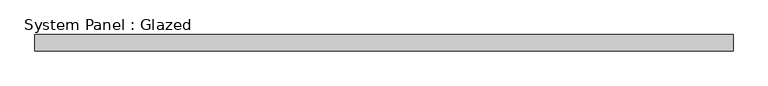
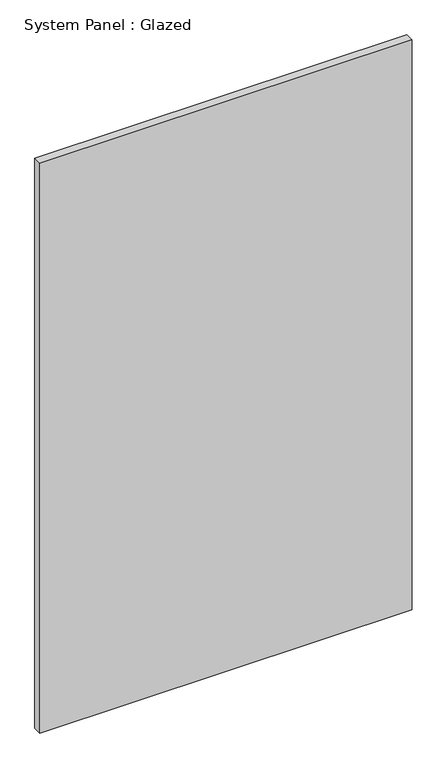
"""IFC4 building model written with IfcOpenShell, lengths in millimetres: plate geometry, System Panel : Glazed."""

from ifc_helpers import new_model, si_unit, origin, origin_with_axes, place, context, project, spatial, polyline, outline, extrude, source, transform, mapped, element, save


def system_panel_glazed_0469dc57(model_context):
    return source(origin(), model_context, "Body", "SweptSolid", [
        extrude(outline(polyline([(534.0, 24.5), (-534.0, 24.5), (-534.0, 49.5), (534.0, 49.5), (534.0, 24.5)])), origin_with_axes(), (0.0, 0.0, 1.0), 1728.8),
    ])


if __name__ == "__main__":
    model = new_model("IFC4")
    model_context = context("Model", 3, world=origin())
    ifc_project = project(units=[si_unit("LENGTHUNIT", "METRE", prefix="MILLI")], contexts=[model_context])
    site = spatial("IfcSite", under=ifc_project)
    building = spatial("IfcBuilding", under=site)
    placement = place(None, origin())
    system_panel_glazed_shape = system_panel_glazed_0469dc57(model_context)
    element("IfcPlate", 1, ObjectType="System Panel : Glazed", at=placement, inside=building, context=model_context, shape_type="MappedRepresentation", body=[
        mapped(system_panel_glazed_shape, transform((0.0, 0.0, 0.0), x_axis=(1.0, 0.0, 0.0), y_axis=(0.0, 1.0, 0.0), z_axis=(0.0, 0.0, 1.0))),
    ])
    save(model, "model.ifc")

# Revit data of these elements
# Type "System Panel : Glazed"
#   Construction Type Id = "GSP4R"
#   Analytic Construction = "1/8 in Pilkington single glazing"
#   Visual Light Transmittance = 0.9
#   Solar Heat Gain Coefficient = 0.86
#   Heat Transfer Coefficient (U) = 6.7069 W/(m²·K)
# Element 1 (IfcPlate, "System Panel : Glazed")
#   Materials on its faces: "Glass"
# Materials
#   "Glass": class "Glass", colour RGB 0 128 192, transparency 0.9, Description = "Soda Lime Glass", Cost = 0
